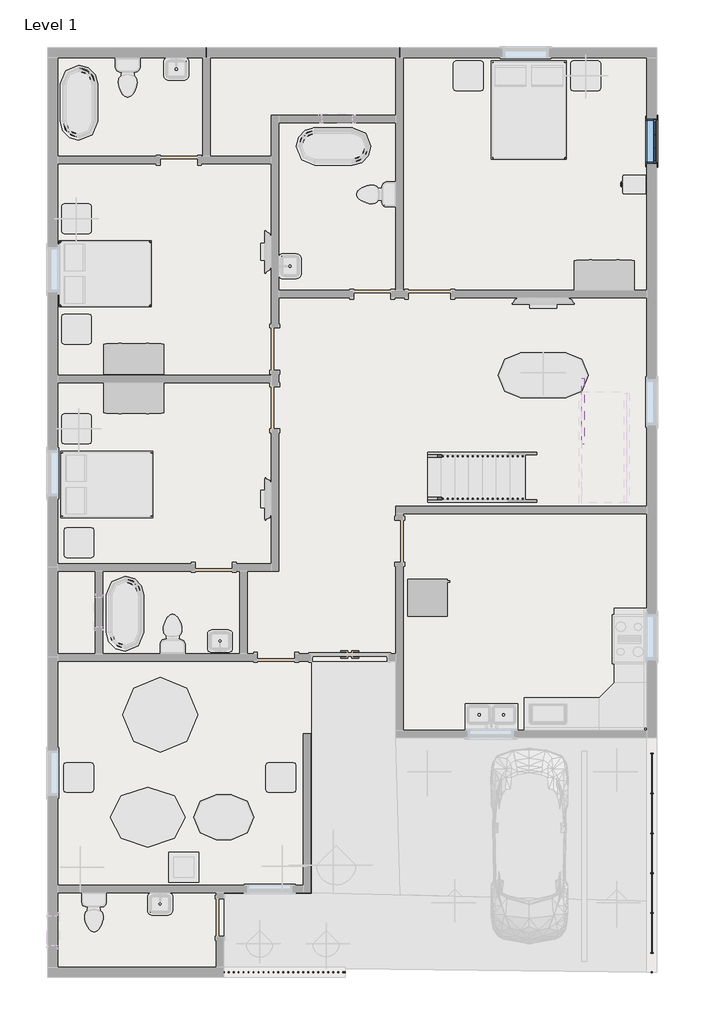
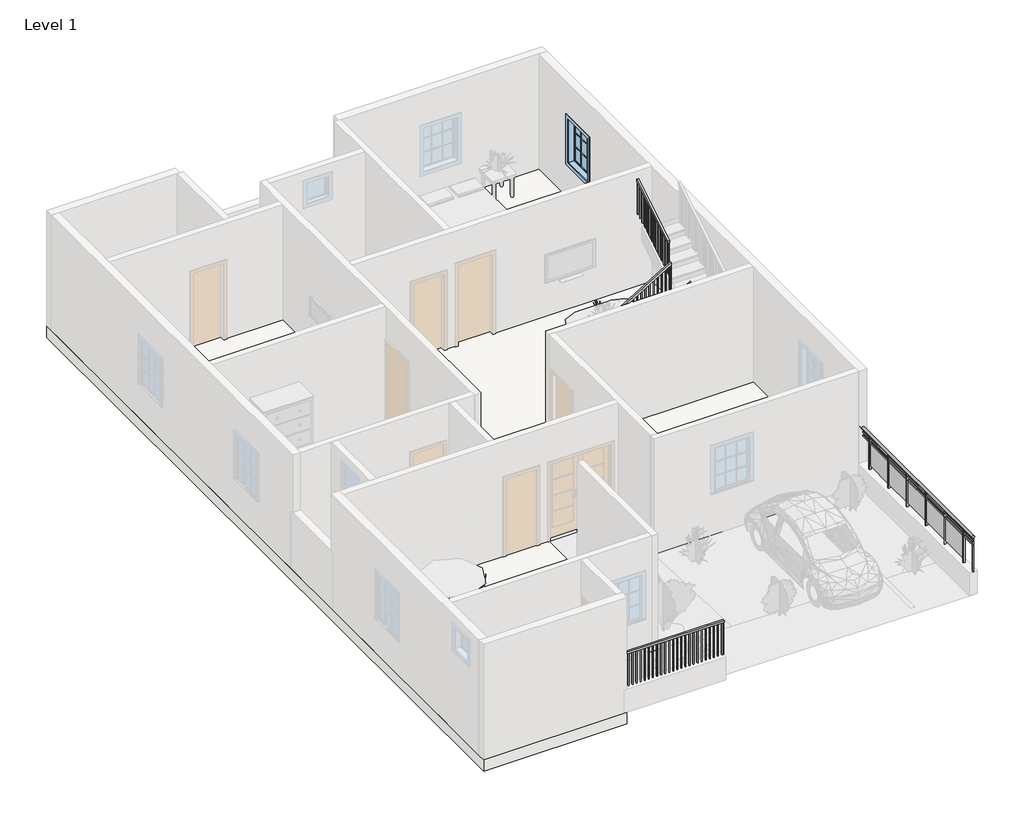
# One storey, part 2 of 3: 5 railings, 1 slab, 1 window.
"""IFC4 building model written with IfcOpenShell, lengths in millimetres."""

from ifc_helpers import new_model, si_unit, point, frame, origin, place, context, project, spatial, polyline, ellipse_curve, trimmed, outline, extrude, transform, mapped, element, save
from ifc_brep_helpers import plane_surface, extruded_surface, advanced_brep
from components import window_29c06734

model = new_model("IFC4")

# Units and contexts
model_context = context("Model", 3, world=origin())
ifc_project = project(units=[si_unit("LENGTHUNIT", "METRE", prefix="MILLI")], contexts=[model_context])

# Site, building, storey
site = spatial("IfcSite", under=ifc_project)
building = spatial("IfcBuilding", under=site)
storey = spatial("IfcBuildingStorey", under=building, Name="Level 1", Elevation=0.0)

# Railings
placement = place(None, origin())
element("IfcRailing", 1, ObjectType="Glass Panel - Bottom Fill", at=placement, inside=storey, context=model_context, shape_type="SolidModel", body=[
    advanced_brep(
    [(197.4210483, -2774.2231522, 1524.0), (121.2210483, -2774.2231522, 1524.0), (197.4210483, -7625.6231522, 1524.0), (121.2210483, -7625.6231522, 1524.0)],
    [
        (0, 1, ellipse_curve(frame((159.3210483, -2774.2231522, 1524.0), z_axis=(0.0, 1.0, 0.0), x_axis=(-1.0, 0.0, 0.0)), 38.1, 28.575)),
        (1, 0, ellipse_curve(frame((159.3210483, -2774.2231522, 1524.0), z_axis=(0.0, 1.0, 0.0), x_axis=(-1.0, 0.0, 0.0)), 38.1, 28.575)),
        (2, 3, ellipse_curve(frame((159.3210483, -7625.6231522, 1524.0), z_axis=(0.0, -1.0, 0.0), x_axis=(-1.0, 0.0, 0.0)), 38.1, 28.575)),
        (3, 2, ellipse_curve(frame((159.3210483, -7625.6231522, 1524.0), z_axis=(0.0, -1.0, 0.0), x_axis=(-1.0, 0.0, 0.0)), 38.1, 28.575)),
        (0, 2),
        (3, 1),
    ],
    [
        plane_surface(frame((159.3210483, -2774.2231522, 1524.0), z_axis=(0.0, 1.0, 0.0), x_axis=(0.0, 0.0, -1.0))),
        plane_surface(frame((159.3210483, -7625.6231522, 1524.0), z_axis=(0.0, -1.0, 0.0), x_axis=(0.0, 0.0, -1.0))),
        extruded_surface(trimmed(ellipse_curve(frame((159.3210483, -7625.6231522, 1524.0), z_axis=(0.0, 1.0, 0.0), x_axis=(-1.0, 0.0, 0.0)), 38.1, 28.575), [point((197.4210483, -7625.6231522, 1524.0))], [point((121.2210483, -7625.6231522, 1524.0))], True, "CARTESIAN"), (0.0, 4851.4, 0.0), 4851.4),
        extruded_surface(trimmed(ellipse_curve(frame((159.3210483, -7625.6231522, 1524.0), z_axis=(0.0, 1.0, 0.0), x_axis=(-1.0, 0.0, 0.0)), 38.1, 28.575), [point((121.2210483, -7625.6231522, 1524.0))], [point((197.4210483, -7625.6231522, 1524.0))], True, "CARTESIAN"), (0.0, 4851.4, 0.0), 4851.4),
    ],
    [
        (0, [[1, 2]]),
        (1, [[3, 4]]),
        (2, [[-1, 5, -4, 6]]),
        (3, [[-2, -6, -3, -5]]),
    ],
),
    extrude(outline(polyline([(146.6210483, -2774.2231522), (172.0210483, -2774.2231522), (172.0210483, -7625.6231522), (146.6210483, -7625.6231522), (146.6210483, -2774.2231522)])), frame((0.0, 0.0, 1409.7), z_axis=(0.0, 0.0, 1.0), x_axis=(1.0, 0.0, 0.0)), (0.0, 0.0, 1.0), 25.4),
    extrude(outline(polyline([(146.6210483, -2774.2231522), (172.0210483, -2774.2231522), (172.0210483, -7625.6231522), (146.6210483, -7625.6231522), (146.6210483, -2774.2231522)])), frame((0.0, 0.0, 1308.1), z_axis=(0.0, 0.0, 1.0), x_axis=(1.0, 0.0, 0.0)), (0.0, 0.0, 1.0), 25.4),
    extrude(outline(polyline([(133.9210483, -7225.5731522), (184.7210483, -7225.5731522), (184.7210483, -7238.2731522), (133.9210483, -7238.2731522), (133.9210483, -7225.5731522)])), frame((0.0, 0.0, 609.6), z_axis=(0.0, 0.0, 1.0), x_axis=(1.0, 0.0, 0.0)), (0.0, 0.0, 1.0), 885.6788223),
    extrude(outline(polyline([(165.8562053, -6419.1231522), (165.8562053, -7231.9231522), (159.5062053, -7231.9231522), (159.5062053, -6419.1231522), (165.8562053, -6419.1231522)])), frame((0.0, 0.0, 711.2), z_axis=(0.0, 0.0, 1.0), x_axis=(1.0, 0.0, 0.0)), (0.0, 0.0, 1.0), 596.9),
    extrude(outline(polyline([(133.9210483, -6412.7731522), (184.7210483, -6412.7731522), (184.7210483, -6425.4731522), (133.9210483, -6425.4731522), (133.9210483, -6412.7731522)])), frame((0.0, 0.0, 609.6), z_axis=(0.0, 0.0, 1.0), x_axis=(1.0, 0.0, 0.0)), (0.0, 0.0, 1.0), 885.6788223),
    extrude(outline(polyline([(165.8562053, -5606.3231522), (165.8562053, -6419.1231522), (159.5062053, -6419.1231522), (159.5062053, -5606.3231522), (165.8562053, -5606.3231522)])), frame((0.0, 0.0, 711.2), z_axis=(0.0, 0.0, 1.0), x_axis=(1.0, 0.0, 0.0)), (0.0, 0.0, 1.0), 596.9),
    extrude(outline(polyline([(133.9210483, -5599.9731522), (184.7210483, -5599.9731522), (184.7210483, -5612.6731522), (133.9210483, -5612.6731522), (133.9210483, -5599.9731522)])), frame((0.0, 0.0, 609.6), z_axis=(0.0, 0.0, 1.0), x_axis=(1.0, 0.0, 0.0)), (0.0, 0.0, 1.0), 885.6788223),
    extrude(outline(polyline([(165.8562053, -4793.5231522), (165.8562053, -5606.3231522), (159.5062053, -5606.3231522), (159.5062053, -4793.5231522), (165.8562053, -4793.5231522)])), frame((0.0, 0.0, 711.2), z_axis=(0.0, 0.0, 1.0), x_axis=(1.0, 0.0, 0.0)), (0.0, 0.0, 1.0), 596.9),
    extrude(outline(polyline([(133.9210483, -4787.1731522), (184.7210483, -4787.1731522), (184.7210483, -4799.8731522), (133.9210483, -4799.8731522), (133.9210483, -4787.1731522)])), frame((0.0, 0.0, 609.6), z_axis=(0.0, 0.0, 1.0), x_axis=(1.0, 0.0, 0.0)), (0.0, 0.0, 1.0), 885.6788223),
    extrude(outline(polyline([(165.8562053, -3980.7231522), (165.8562053, -4793.5231522), (159.5062053, -4793.5231522), (159.5062053, -3980.7231522), (165.8562053, -3980.7231522)])), frame((0.0, 0.0, 711.2), z_axis=(0.0, 0.0, 1.0), x_axis=(1.0, 0.0, 0.0)), (0.0, 0.0, 1.0), 596.9),
    extrude(outline(polyline([(133.9210483, -3974.3731522), (184.7210483, -3974.3731522), (184.7210483, -3987.0731522), (133.9210483, -3987.0731522), (133.9210483, -3974.3731522)])), frame((0.0, 0.0, 609.6), z_axis=(0.0, 0.0, 1.0), x_axis=(1.0, 0.0, 0.0)), (0.0, 0.0, 1.0), 885.6788223),
    extrude(outline(polyline([(165.8562053, -3167.9231522), (165.8562053, -3980.7231522), (159.5062053, -3980.7231522), (159.5062053, -3167.9231522), (165.8562053, -3167.9231522)])), frame((0.0, 0.0, 711.2), z_axis=(0.0, 0.0, 1.0), x_axis=(1.0, 0.0, 0.0)), (0.0, 0.0, 1.0), 596.9),
    extrude(outline(polyline([(133.9210483, -3161.5731522), (184.7210483, -3161.5731522), (184.7210483, -3174.2731522), (133.9210483, -3174.2731522), (133.9210483, -3161.5731522)])), frame((0.0, 0.0, 609.6), z_axis=(0.0, 0.0, 1.0), x_axis=(1.0, 0.0, 0.0)), (0.0, 0.0, 1.0), 885.6788223),
    extrude(outline(polyline([(149.7960483, -7612.9231522), (168.8460483, -7612.9231522), (168.8460483, -7631.9731522), (149.7960483, -7631.9731522), (149.7960483, -7612.9231522)])), frame((0.0, 0.0, 609.6), z_axis=(0.0, 0.0, 1.0), x_axis=(1.0, 0.0, 0.0)), (0.0, 0.0, 1.0), 885.6788223),
    extrude(outline(polyline([(149.7960483, -2767.8731522), (168.8460483, -2767.8731522), (168.8460483, -2786.9231522), (149.7960483, -2786.9231522), (149.7960483, -2767.8731522)])), frame((0.0, 0.0, 609.6), z_axis=(0.0, 0.0, 1.0), x_axis=(1.0, 0.0, 0.0)), (0.0, 0.0, 1.0), 885.6788223),
])
element("IfcRailing", 2, ObjectType="Handrail - Rectangular", at=placement, inside=storey, context=model_context, shape_type="SweptSolid", body=[
    extrude(outline(polyline([(1083.7333333, -4400.7663486), (1024.3318731, -4400.7663486), (2886.9985397, -1327.3663486), (2946.4, -1327.3663486), (1083.7333333, -4400.7663486)])), frame((0.0, 1993.3117215, 0.0), z_axis=(0.0, 1.0, 0.0), x_axis=(0.0, 0.0, 1.0)), (0.0, 0.0, 1.0), 50.8),
    extrude(outline(polyline([(2877.3773276, -1343.2413486), (2865.8318731, -1362.2913486), (1862.6666667, -1362.2913486), (1862.6666667, -1343.2413486), (2877.3773276, -1343.2413486)])), frame((0.0, 2009.1867215, 0.0), z_axis=(0.0, 1.0, 0.0), x_axis=(0.0, 0.0, 1.0)), (0.0, 0.0, 1.0), 19.05),
    extrude(outline(polyline([(2815.80157, -1444.8413486), (2804.2561155, -1463.8913486), (1862.6666667, -1463.8913486), (1862.6666667, -1444.8413486), (2815.80157, -1444.8413486)])), frame((0.0, 2009.1867215, 0.0), z_axis=(0.0, 1.0, 0.0), x_axis=(0.0, 0.0, 1.0)), (0.0, 0.0, 1.0), 19.05),
    extrude(outline(polyline([(2754.2258125, -1546.4413486), (2742.6803579, -1565.4913486), (1862.6666667, -1565.4913486), (1862.6666667, -1546.4413486), (2754.2258125, -1546.4413486)])), frame((0.0, 2009.1867215, 0.0), z_axis=(0.0, 1.0, 0.0), x_axis=(0.0, 0.0, 1.0)), (0.0, 0.0, 1.0), 19.05),
    extrude(outline(polyline([(2692.6500549, -1648.0413486), (2681.1046004, -1667.0913486), (1693.3333333, -1667.0913486), (1693.3333333, -1648.0413486), (2692.6500549, -1648.0413486)])), frame((0.0, 2009.1867215, 0.0), z_axis=(0.0, 1.0, 0.0), x_axis=(0.0, 0.0, 1.0)), (0.0, 0.0, 1.0), 19.05),
    extrude(outline(polyline([(2631.0742973, -1749.6413486), (2619.5288428, -1768.6913486), (1693.3333333, -1768.6913486), (1693.3333333, -1749.6413486), (2631.0742973, -1749.6413486)])), frame((0.0, 2009.1867215, 0.0), z_axis=(0.0, 1.0, 0.0), x_axis=(0.0, 0.0, 1.0)), (0.0, 0.0, 1.0), 19.05),
    extrude(outline(polyline([(2569.4985397, -1851.2413486), (2557.9530852, -1870.2913486), (1693.3333333, -1870.2913486), (1693.3333333, -1851.2413486), (2569.4985397, -1851.2413486)])), frame((0.0, 2009.1867215, 0.0), z_axis=(0.0, 1.0, 0.0), x_axis=(0.0, 0.0, 1.0)), (0.0, 0.0, 1.0), 19.05),
    extrude(outline(polyline([(2507.9227822, -1952.8413486), (2496.3773276, -1971.8913486), (1524.0, -1971.8913486), (1524.0, -1952.8413486), (2507.9227822, -1952.8413486)])), frame((0.0, 2009.1867215, 0.0), z_axis=(0.0, 1.0, 0.0), x_axis=(0.0, 0.0, 1.0)), (0.0, 0.0, 1.0), 19.05),
    extrude(outline(polyline([(2446.3470246, -2054.4413486), (2434.80157, -2073.4913486), (1524.0, -2073.4913486), (1524.0, -2054.4413486), (2446.3470246, -2054.4413486)])), frame((0.0, 2009.1867215, 0.0), z_axis=(0.0, 1.0, 0.0), x_axis=(0.0, 0.0, 1.0)), (0.0, 0.0, 1.0), 19.05),
    extrude(outline(polyline([(2384.771267, -2156.0413486), (2373.2258125, -2175.0913486), (1524.0, -2175.0913486), (1524.0, -2156.0413486), (2384.771267, -2156.0413486)])), frame((0.0, 2009.1867215, 0.0), z_axis=(0.0, 1.0, 0.0), x_axis=(0.0, 0.0, 1.0)), (0.0, 0.0, 1.0), 19.05),
    extrude(outline(polyline([(2323.1955094, -2257.6413486), (2311.6500549, -2276.6913486), (1354.6666667, -2276.6913486), (1354.6666667, -2257.6413486), (2323.1955094, -2257.6413486)])), frame((0.0, 2009.1867215, 0.0), z_axis=(0.0, 1.0, 0.0), x_axis=(0.0, 0.0, 1.0)), (0.0, 0.0, 1.0), 19.05),
    extrude(outline(polyline([(2261.6197519, -2359.2413486), (2250.0742973, -2378.2913486), (1354.6666667, -2378.2913486), (1354.6666667, -2359.2413486), (2261.6197519, -2359.2413486)])), frame((0.0, 2009.1867215, 0.0), z_axis=(0.0, 1.0, 0.0), x_axis=(0.0, 0.0, 1.0)), (0.0, 0.0, 1.0), 19.05),
    extrude(outline(polyline([(2200.0439943, -2460.8413486), (2188.4985397, -2479.8913486), (1185.3333333, -2479.8913486), (1185.3333333, -2460.8413486), (2200.0439943, -2460.8413486)])), frame((0.0, 2009.1867215, 0.0), z_axis=(0.0, 1.0, 0.0), x_axis=(0.0, 0.0, 1.0)), (0.0, 0.0, 1.0), 19.05),
    extrude(outline(polyline([(2138.4682367, -2562.4413486), (2126.9227822, -2581.4913486), (1185.3333333, -2581.4913486), (1185.3333333, -2562.4413486), (2138.4682367, -2562.4413486)])), frame((0.0, 2009.1867215, 0.0), z_axis=(0.0, 1.0, 0.0), x_axis=(0.0, 0.0, 1.0)), (0.0, 0.0, 1.0), 19.05),
    extrude(outline(polyline([(2076.8924791, -2664.0413486), (2065.3470246, -2683.0913486), (1185.3333333, -2683.0913486), (1185.3333333, -2664.0413486), (2076.8924791, -2664.0413486)])), frame((0.0, 2009.1867215, 0.0), z_axis=(0.0, 1.0, 0.0), x_axis=(0.0, 0.0, 1.0)), (0.0, 0.0, 1.0), 19.05),
    extrude(outline(polyline([(2015.3167216, -2765.6413486), (2003.771267, -2784.6913486), (1016.0, -2784.6913486), (1016.0, -2765.6413486), (2015.3167216, -2765.6413486)])), frame((0.0, 2009.1867215, 0.0), z_axis=(0.0, 1.0, 0.0), x_axis=(0.0, 0.0, 1.0)), (0.0, 0.0, 1.0), 19.05),
    extrude(outline(polyline([(1953.740964, -2867.2413486), (1942.1955094, -2886.2913486), (1016.0, -2886.2913486), (1016.0, -2867.2413486), (1953.740964, -2867.2413486)])), frame((0.0, 2009.1867215, 0.0), z_axis=(0.0, 1.0, 0.0), x_axis=(0.0, 0.0, 1.0)), (0.0, 0.0, 1.0), 19.05),
    extrude(outline(polyline([(1892.1652064, -2968.8413486), (1880.6197519, -2987.8913486), (1016.0, -2987.8913486), (1016.0, -2968.8413486), (1892.1652064, -2968.8413486)])), frame((0.0, 2009.1867215, 0.0), z_axis=(0.0, 1.0, 0.0), x_axis=(0.0, 0.0, 1.0)), (0.0, 0.0, 1.0), 19.05),
    extrude(outline(polyline([(1830.5894488, -3070.4413486), (1819.0439943, -3089.4913486), (846.6666667, -3089.4913486), (846.6666667, -3070.4413486), (1830.5894488, -3070.4413486)])), frame((0.0, 2009.1867215, 0.0), z_axis=(0.0, 1.0, 0.0), x_axis=(0.0, 0.0, 1.0)), (0.0, 0.0, 1.0), 19.05),
    extrude(outline(polyline([(1769.0136913, -3172.0413486), (1757.4682367, -3191.0913486), (846.6666667, -3191.0913486), (846.6666667, -3172.0413486), (1769.0136913, -3172.0413486)])), frame((0.0, 2009.1867215, 0.0), z_axis=(0.0, 1.0, 0.0), x_axis=(0.0, 0.0, 1.0)), (0.0, 0.0, 1.0), 19.05),
    extrude(outline(polyline([(1707.4379337, -3273.6413486), (1695.8924791, -3292.6913486), (846.6666667, -3292.6913486), (846.6666667, -3273.6413486), (1707.4379337, -3273.6413486)])), frame((0.0, 2009.1867215, 0.0), z_axis=(0.0, 1.0, 0.0), x_axis=(0.0, 0.0, 1.0)), (0.0, 0.0, 1.0), 19.05),
    extrude(outline(polyline([(1645.8621761, -3375.2413486), (1634.3167216, -3394.2913486), (677.3333333, -3394.2913486), (677.3333333, -3375.2413486), (1645.8621761, -3375.2413486)])), frame((0.0, 2009.1867215, 0.0), z_axis=(0.0, 1.0, 0.0), x_axis=(0.0, 0.0, 1.0)), (0.0, 0.0, 1.0), 19.05),
    extrude(outline(polyline([(1584.2864185, -3476.8413486), (1572.740964, -3495.8913486), (677.3333333, -3495.8913486), (677.3333333, -3476.8413486), (1584.2864185, -3476.8413486)])), frame((0.0, 2009.1867215, 0.0), z_axis=(0.0, 1.0, 0.0), x_axis=(0.0, 0.0, 1.0)), (0.0, 0.0, 1.0), 19.05),
    extrude(outline(polyline([(1522.710661, -3578.4413486), (1511.1652064, -3597.4913486), (508.0, -3597.4913486), (508.0, -3578.4413486), (1522.710661, -3578.4413486)])), frame((0.0, 2009.1867215, 0.0), z_axis=(0.0, 1.0, 0.0), x_axis=(0.0, 0.0, 1.0)), (0.0, 0.0, 1.0), 19.05),
    extrude(outline(polyline([(1461.1349034, -3680.0413486), (1449.5894488, -3699.0913486), (508.0, -3699.0913486), (508.0, -3680.0413486), (1461.1349034, -3680.0413486)])), frame((0.0, 2009.1867215, 0.0), z_axis=(0.0, 1.0, 0.0), x_axis=(0.0, 0.0, 1.0)), (0.0, 0.0, 1.0), 19.05),
    extrude(outline(polyline([(1399.5591458, -3781.6413486), (1388.0136913, -3800.6913486), (508.0, -3800.6913486), (508.0, -3781.6413486), (1399.5591458, -3781.6413486)])), frame((0.0, 2009.1867215, 0.0), z_axis=(0.0, 1.0, 0.0), x_axis=(0.0, 0.0, 1.0)), (0.0, 0.0, 1.0), 19.05),
    extrude(outline(polyline([(1337.9833882, -3883.2413486), (1326.4379337, -3902.2913486), (338.6666667, -3902.2913486), (338.6666667, -3883.2413486), (1337.9833882, -3883.2413486)])), frame((0.0, 2009.1867215, 0.0), z_axis=(0.0, 1.0, 0.0), x_axis=(0.0, 0.0, 1.0)), (0.0, 0.0, 1.0), 19.05),
    extrude(outline(polyline([(1276.4076307, -3984.8413486), (1264.8621761, -4003.8913486), (338.6666667, -4003.8913486), (338.6666667, -3984.8413486), (1276.4076307, -3984.8413486)])), frame((0.0, 2009.1867215, 0.0), z_axis=(0.0, 1.0, 0.0), x_axis=(0.0, 0.0, 1.0)), (0.0, 0.0, 1.0), 19.05),
    extrude(outline(polyline([(1214.8318731, -4086.4413486), (1203.2864185, -4105.4913486), (338.6666667, -4105.4913486), (338.6666667, -4086.4413486), (1214.8318731, -4086.4413486)])), frame((0.0, 2009.1867215, 0.0), z_axis=(0.0, 1.0, 0.0), x_axis=(0.0, 0.0, 1.0)), (0.0, 0.0, 1.0), 19.05),
    extrude(outline(polyline([(1153.2561155, -4188.0413486), (1141.710661, -4207.0913486), (169.3333333, -4207.0913486), (169.3333333, -4188.0413486), (1153.2561155, -4188.0413486)])), frame((0.0, 2009.1867215, 0.0), z_axis=(0.0, 1.0, 0.0), x_axis=(0.0, 0.0, 1.0)), (0.0, 0.0, 1.0), 19.05),
    extrude(outline(polyline([(1091.6803579, -4289.6413486), (1080.1349034, -4308.6913486), (169.3333333, -4308.6913486), (169.3333333, -4289.6413486), (1091.6803579, -4289.6413486)])), frame((0.0, 2009.1867215, 0.0), z_axis=(0.0, 1.0, 0.0), x_axis=(0.0, 0.0, 1.0)), (0.0, 0.0, 1.0), 19.05),
    extrude(outline(polyline([(2886.9985397, -1327.3663486), (2875.4530852, -1346.4163486), (1862.6666667, -1346.4163486), (1862.6666667, -1327.3663486), (2886.9985397, -1327.3663486)])), frame((0.0, 2009.1867215, 0.0), z_axis=(0.0, 1.0, 0.0), x_axis=(0.0, 0.0, 1.0)), (0.0, 0.0, 1.0), 19.05),
    extrude(outline(polyline([(1035.8773276, -4381.7163486), (1024.3318731, -4400.7663486), (169.3333333, -4400.7663486), (169.3333333, -4381.7163486), (1035.8773276, -4381.7163486)])), frame((0.0, 2009.1867215, 0.0), z_axis=(0.0, 1.0, 0.0), x_axis=(0.0, 0.0, 1.0)), (0.0, 0.0, 1.0), 19.05),
])
element("IfcRailing", 3, ObjectType="Handrail - Rectangular", at=placement, inside=storey, context=model_context, shape_type="SweptSolid", body=[
    extrude(outline(polyline([(1083.7333333, -4400.7663486), (1024.3318731, -4400.7663486), (2886.9985397, -1327.3663486), (2946.4, -1327.3663486), (1083.7333333, -4400.7663486)])), frame((0.0, 2856.9117215, 0.0), z_axis=(0.0, 1.0, 0.0), x_axis=(0.0, 0.0, 1.0)), (0.0, 0.0, 1.0), 50.8),
    extrude(outline(polyline([(2865.8318731, -1362.2913486), (1862.6666667, -1362.2913486), (1862.6666667, -1343.2413486), (2877.3773276, -1343.2413486), (2865.8318731, -1362.2913486)])), frame((0.0, 2872.7867215, 0.0), z_axis=(0.0, 1.0, 0.0), x_axis=(0.0, 0.0, 1.0)), (0.0, 0.0, 1.0), 19.05),
    extrude(outline(polyline([(2804.2561155, -1463.8913486), (1862.6666667, -1463.8913486), (1862.6666667, -1444.8413486), (2815.80157, -1444.8413486), (2804.2561155, -1463.8913486)])), frame((0.0, 2872.7867215, 0.0), z_axis=(0.0, 1.0, 0.0), x_axis=(0.0, 0.0, 1.0)), (0.0, 0.0, 1.0), 19.05),
    extrude(outline(polyline([(2742.6803579, -1565.4913486), (1862.6666667, -1565.4913486), (1862.6666667, -1546.4413486), (2754.2258125, -1546.4413486), (2742.6803579, -1565.4913486)])), frame((0.0, 2872.7867215, 0.0), z_axis=(0.0, 1.0, 0.0), x_axis=(0.0, 0.0, 1.0)), (0.0, 0.0, 1.0), 19.05),
    extrude(outline(polyline([(2681.1046004, -1667.0913486), (1693.3333333, -1667.0913486), (1693.3333333, -1648.0413486), (2692.6500549, -1648.0413486), (2681.1046004, -1667.0913486)])), frame((0.0, 2872.7867215, 0.0), z_axis=(0.0, 1.0, 0.0), x_axis=(0.0, 0.0, 1.0)), (0.0, 0.0, 1.0), 19.05),
    extrude(outline(polyline([(2619.5288428, -1768.6913486), (1693.3333333, -1768.6913486), (1693.3333333, -1749.6413486), (2631.0742973, -1749.6413486), (2619.5288428, -1768.6913486)])), frame((0.0, 2872.7867215, 0.0), z_axis=(0.0, 1.0, 0.0), x_axis=(0.0, 0.0, 1.0)), (0.0, 0.0, 1.0), 19.05),
    extrude(outline(polyline([(2557.9530852, -1870.2913486), (1693.3333333, -1870.2913486), (1693.3333333, -1851.2413486), (2569.4985397, -1851.2413486), (2557.9530852, -1870.2913486)])), frame((0.0, 2872.7867215, 0.0), z_axis=(0.0, 1.0, 0.0), x_axis=(0.0, 0.0, 1.0)), (0.0, 0.0, 1.0), 19.05),
    extrude(outline(polyline([(2496.3773276, -1971.8913486), (1524.0, -1971.8913486), (1524.0, -1952.8413486), (2507.9227822, -1952.8413486), (2496.3773276, -1971.8913486)])), frame((0.0, 2872.7867215, 0.0), z_axis=(0.0, 1.0, 0.0), x_axis=(0.0, 0.0, 1.0)), (0.0, 0.0, 1.0), 19.05),
    extrude(outline(polyline([(2434.80157, -2073.4913486), (1524.0, -2073.4913486), (1524.0, -2054.4413486), (2446.3470246, -2054.4413486), (2434.80157, -2073.4913486)])), frame((0.0, 2872.7867215, 0.0), z_axis=(0.0, 1.0, 0.0), x_axis=(0.0, 0.0, 1.0)), (0.0, 0.0, 1.0), 19.05),
    extrude(outline(polyline([(2373.2258125, -2175.0913486), (1524.0, -2175.0913486), (1524.0, -2156.0413486), (2384.771267, -2156.0413486), (2373.2258125, -2175.0913486)])), frame((0.0, 2872.7867215, 0.0), z_axis=(0.0, 1.0, 0.0), x_axis=(0.0, 0.0, 1.0)), (0.0, 0.0, 1.0), 19.05),
    extrude(outline(polyline([(2311.6500549, -2276.6913486), (1354.6666667, -2276.6913486), (1354.6666667, -2257.6413486), (2323.1955094, -2257.6413486), (2311.6500549, -2276.6913486)])), frame((0.0, 2872.7867215, 0.0), z_axis=(0.0, 1.0, 0.0), x_axis=(0.0, 0.0, 1.0)), (0.0, 0.0, 1.0), 19.05),
    extrude(outline(polyline([(2250.0742973, -2378.2913486), (1354.6666667, -2378.2913486), (1354.6666667, -2359.2413486), (2261.6197519, -2359.2413486), (2250.0742973, -2378.2913486)])), frame((0.0, 2872.7867215, 0.0), z_axis=(0.0, 1.0, 0.0), x_axis=(0.0, 0.0, 1.0)), (0.0, 0.0, 1.0), 19.05),
    extrude(outline(polyline([(2188.4985397, -2479.8913486), (1185.3333333, -2479.8913486), (1185.3333333, -2460.8413486), (2200.0439943, -2460.8413486), (2188.4985397, -2479.8913486)])), frame((0.0, 2872.7867215, 0.0), z_axis=(0.0, 1.0, 0.0), x_axis=(0.0, 0.0, 1.0)), (0.0, 0.0, 1.0), 19.05),
    extrude(outline(polyline([(2126.9227822, -2581.4913486), (1185.3333333, -2581.4913486), (1185.3333333, -2562.4413486), (2138.4682367, -2562.4413486), (2126.9227822, -2581.4913486)])), frame((0.0, 2872.7867215, 0.0), z_axis=(0.0, 1.0, 0.0), x_axis=(0.0, 0.0, 1.0)), (0.0, 0.0, 1.0), 19.05),
    extrude(outline(polyline([(2065.3470246, -2683.0913486), (1185.3333333, -2683.0913486), (1185.3333333, -2664.0413486), (2076.8924791, -2664.0413486), (2065.3470246, -2683.0913486)])), frame((0.0, 2872.7867215, 0.0), z_axis=(0.0, 1.0, 0.0), x_axis=(0.0, 0.0, 1.0)), (0.0, 0.0, 1.0), 19.05),
    extrude(outline(polyline([(2003.771267, -2784.6913486), (1016.0, -2784.6913486), (1016.0, -2765.6413486), (2015.3167216, -2765.6413486), (2003.771267, -2784.6913486)])), frame((0.0, 2872.7867215, 0.0), z_axis=(0.0, 1.0, 0.0), x_axis=(0.0, 0.0, 1.0)), (0.0, 0.0, 1.0), 19.05),
    extrude(outline(polyline([(1942.1955094, -2886.2913486), (1016.0, -2886.2913486), (1016.0, -2867.2413486), (1953.740964, -2867.2413486), (1942.1955094, -2886.2913486)])), frame((0.0, 2872.7867215, 0.0), z_axis=(0.0, 1.0, 0.0), x_axis=(0.0, 0.0, 1.0)), (0.0, 0.0, 1.0), 19.05),
    extrude(outline(polyline([(1880.6197519, -2987.8913486), (1016.0, -2987.8913486), (1016.0, -2968.8413486), (1892.1652064, -2968.8413486), (1880.6197519, -2987.8913486)])), frame((0.0, 2872.7867215, 0.0), z_axis=(0.0, 1.0, 0.0), x_axis=(0.0, 0.0, 1.0)), (0.0, 0.0, 1.0), 19.05),
    extrude(outline(polyline([(1819.0439943, -3089.4913486), (846.6666667, -3089.4913486), (846.6666667, -3070.4413486), (1830.5894488, -3070.4413486), (1819.0439943, -3089.4913486)])), frame((0.0, 2872.7867215, 0.0), z_axis=(0.0, 1.0, 0.0), x_axis=(0.0, 0.0, 1.0)), (0.0, 0.0, 1.0), 19.05),
    extrude(outline(polyline([(1757.4682367, -3191.0913486), (846.6666667, -3191.0913486), (846.6666667, -3172.0413486), (1769.0136913, -3172.0413486), (1757.4682367, -3191.0913486)])), frame((0.0, 2872.7867215, 0.0), z_axis=(0.0, 1.0, 0.0), x_axis=(0.0, 0.0, 1.0)), (0.0, 0.0, 1.0), 19.05),
    extrude(outline(polyline([(1695.8924791, -3292.6913486), (846.6666667, -3292.6913486), (846.6666667, -3273.6413486), (1707.4379337, -3273.6413486), (1695.8924791, -3292.6913486)])), frame((0.0, 2872.7867215, 0.0), z_axis=(0.0, 1.0, 0.0), x_axis=(0.0, 0.0, 1.0)), (0.0, 0.0, 1.0), 19.05),
    extrude(outline(polyline([(1634.3167216, -3394.2913486), (677.3333333, -3394.2913486), (677.3333333, -3375.2413486), (1645.8621761, -3375.2413486), (1634.3167216, -3394.2913486)])), frame((0.0, 2872.7867215, 0.0), z_axis=(0.0, 1.0, 0.0), x_axis=(0.0, 0.0, 1.0)), (0.0, 0.0, 1.0), 19.05),
    extrude(outline(polyline([(1572.740964, -3495.8913486), (677.3333333, -3495.8913486), (677.3333333, -3476.8413486), (1584.2864185, -3476.8413486), (1572.740964, -3495.8913486)])), frame((0.0, 2872.7867215, 0.0), z_axis=(0.0, 1.0, 0.0), x_axis=(0.0, 0.0, 1.0)), (0.0, 0.0, 1.0), 19.05),
    extrude(outline(polyline([(1511.1652064, -3597.4913486), (508.0, -3597.4913486), (508.0, -3578.4413486), (1522.710661, -3578.4413486), (1511.1652064, -3597.4913486)])), frame((0.0, 2872.7867215, 0.0), z_axis=(0.0, 1.0, 0.0), x_axis=(0.0, 0.0, 1.0)), (0.0, 0.0, 1.0), 19.05),
    extrude(outline(polyline([(1449.5894488, -3699.0913486), (508.0, -3699.0913486), (508.0, -3680.0413486), (1461.1349034, -3680.0413486), (1449.5894488, -3699.0913486)])), frame((0.0, 2872.7867215, 0.0), z_axis=(0.0, 1.0, 0.0), x_axis=(0.0, 0.0, 1.0)), (0.0, 0.0, 1.0), 19.05),
    extrude(outline(polyline([(1388.0136913, -3800.6913486), (508.0, -3800.6913486), (508.0, -3781.6413486), (1399.5591458, -3781.6413486), (1388.0136913, -3800.6913486)])), frame((0.0, 2872.7867215, 0.0), z_axis=(0.0, 1.0, 0.0), x_axis=(0.0, 0.0, 1.0)), (0.0, 0.0, 1.0), 19.05),
    extrude(outline(polyline([(1326.4379337, -3902.2913486), (338.6666667, -3902.2913486), (338.6666667, -3883.2413486), (1337.9833882, -3883.2413486), (1326.4379337, -3902.2913486)])), frame((0.0, 2872.7867215, 0.0), z_axis=(0.0, 1.0, 0.0), x_axis=(0.0, 0.0, 1.0)), (0.0, 0.0, 1.0), 19.05),
    extrude(outline(polyline([(1264.8621761, -4003.8913486), (338.6666667, -4003.8913486), (338.6666667, -3984.8413486), (1276.4076307, -3984.8413486), (1264.8621761, -4003.8913486)])), frame((0.0, 2872.7867215, 0.0), z_axis=(0.0, 1.0, 0.0), x_axis=(0.0, 0.0, 1.0)), (0.0, 0.0, 1.0), 19.05),
    extrude(outline(polyline([(1203.2864185, -4105.4913486), (338.6666667, -4105.4913486), (338.6666667, -4086.4413486), (1214.8318731, -4086.4413486), (1203.2864185, -4105.4913486)])), frame((0.0, 2872.7867215, 0.0), z_axis=(0.0, 1.0, 0.0), x_axis=(0.0, 0.0, 1.0)), (0.0, 0.0, 1.0), 19.05),
    extrude(outline(polyline([(1141.710661, -4207.0913486), (169.3333333, -4207.0913486), (169.3333333, -4188.0413486), (1153.2561155, -4188.0413486), (1141.710661, -4207.0913486)])), frame((0.0, 2872.7867215, 0.0), z_axis=(0.0, 1.0, 0.0), x_axis=(0.0, 0.0, 1.0)), (0.0, 0.0, 1.0), 19.05),
    extrude(outline(polyline([(1080.1349034, -4308.6913486), (169.3333333, -4308.6913486), (169.3333333, -4289.6413486), (1091.6803579, -4289.6413486), (1080.1349034, -4308.6913486)])), frame((0.0, 2872.7867215, 0.0), z_axis=(0.0, 1.0, 0.0), x_axis=(0.0, 0.0, 1.0)), (0.0, 0.0, 1.0), 19.05),
    extrude(outline(polyline([(2875.4530852, -1346.4163486), (1862.6666667, -1346.4163486), (1862.6666667, -1327.3663486), (2886.9985397, -1327.3663486), (2875.4530852, -1346.4163486)])), frame((0.0, 2872.7867215, 0.0), z_axis=(0.0, 1.0, 0.0), x_axis=(0.0, 0.0, 1.0)), (0.0, 0.0, 1.0), 19.05),
    extrude(outline(polyline([(1024.3318731, -4400.7663486), (169.3333333, -4400.7663486), (169.3333333, -4381.7163486), (1035.8773276, -4381.7163486), (1024.3318731, -4400.7663486)])), frame((0.0, 2872.7867215, 0.0), z_axis=(0.0, 1.0, 0.0), x_axis=(0.0, 0.0, 1.0)), (0.0, 0.0, 1.0), 19.05),
])
element("IfcRailing", 4, ObjectType="Handrail - Rectangular", at=placement, inside=storey, context=model_context, shape_type="SweptSolid", body=[
    extrude(outline(polyline([(3124.388941, 3271.7078476), (3124.388941, 3331.1093079), (4470.588941, 4146.9880957), (4470.588941, 4087.5866355), (3124.388941, 3271.7078476)])), frame((-1263.0789517, 0.0, 0.0), z_axis=(1.0, 0.0, 0.0), x_axis=(0.0, 1.0, 0.0)), (0.0, 0.0, 1.0), 50.8),
    extrude(outline(polyline([(3140.263941, 3281.4682367), (3159.313941, 3293.0136913), (3159.313941, 2370.6666667), (3140.263941, 2370.6666667), (3140.263941, 3281.4682367)])), frame((-1247.2039517, 0.0, 0.0), z_axis=(1.0, 0.0, 0.0), x_axis=(0.0, 1.0, 0.0)), (0.0, 0.0, 1.0), 19.05),
    extrude(outline(polyline([(3241.863941, 3343.0439943), (3260.913941, 3354.5894488), (3260.913941, 2370.6666667), (3241.863941, 2370.6666667), (3241.863941, 3343.0439943)])), frame((-1247.2039517, 0.0, 0.0), z_axis=(1.0, 0.0, 0.0), x_axis=(0.0, 1.0, 0.0)), (0.0, 0.0, 1.0), 19.05),
    extrude(outline(polyline([(3343.463941, 3404.6197519), (3362.513941, 3416.1652064), (3362.513941, 2540.0), (3343.463941, 2540.0), (3343.463941, 3404.6197519)])), frame((-1247.2039517, 0.0, 0.0), z_axis=(1.0, 0.0, 0.0), x_axis=(0.0, 1.0, 0.0)), (0.0, 0.0, 1.0), 19.05),
    extrude(outline(polyline([(3445.063941, 3466.1955094), (3464.113941, 3477.740964), (3464.113941, 2540.0), (3445.063941, 2540.0), (3445.063941, 3466.1955094)])), frame((-1247.2039517, 0.0, 0.0), z_axis=(1.0, 0.0, 0.0), x_axis=(0.0, 1.0, 0.0)), (0.0, 0.0, 1.0), 19.05),
    extrude(outline(polyline([(3546.663941, 3527.771267), (3565.713941, 3539.3167216), (3565.713941, 2540.0), (3546.663941, 2540.0), (3546.663941, 3527.771267)])), frame((-1247.2039517, 0.0, 0.0), z_axis=(1.0, 0.0, 0.0), x_axis=(0.0, 1.0, 0.0)), (0.0, 0.0, 1.0), 19.05),
    extrude(outline(polyline([(3648.263941, 3589.3470246), (3667.313941, 3600.8924791), (3667.313941, 2709.3333333), (3648.263941, 2709.3333333), (3648.263941, 3589.3470246)])), frame((-1247.2039517, 0.0, 0.0), z_axis=(1.0, 0.0, 0.0), x_axis=(0.0, 1.0, 0.0)), (0.0, 0.0, 1.0), 19.05),
    extrude(outline(polyline([(3749.863941, 3650.9227822), (3768.913941, 3662.4682367), (3768.913941, 2709.3333333), (3749.863941, 2709.3333333), (3749.863941, 3650.9227822)])), frame((-1247.2039517, 0.0, 0.0), z_axis=(1.0, 0.0, 0.0), x_axis=(0.0, 1.0, 0.0)), (0.0, 0.0, 1.0), 19.05),
    extrude(outline(polyline([(3851.463941, 3712.4985397), (3870.513941, 3724.0439943), (3870.513941, 2709.3333333), (3851.463941, 2709.3333333), (3851.463941, 3712.4985397)])), frame((-1247.2039517, 0.0, 0.0), z_axis=(1.0, 0.0, 0.0), x_axis=(0.0, 1.0, 0.0)), (0.0, 0.0, 1.0), 19.05),
    extrude(outline(polyline([(3953.063941, 3774.0742973), (3972.113941, 3785.6197519), (3972.113941, 2878.6666667), (3953.063941, 2878.6666667), (3953.063941, 3774.0742973)])), frame((-1247.2039517, 0.0, 0.0), z_axis=(1.0, 0.0, 0.0), x_axis=(0.0, 1.0, 0.0)), (0.0, 0.0, 1.0), 19.05),
    extrude(outline(polyline([(4054.663941, 3835.6500549), (4073.713941, 3847.1955094), (4073.713941, 2878.6666667), (4054.663941, 2878.6666667), (4054.663941, 3835.6500549)])), frame((-1247.2039517, 0.0, 0.0), z_axis=(1.0, 0.0, 0.0), x_axis=(0.0, 1.0, 0.0)), (0.0, 0.0, 1.0), 19.05),
    extrude(outline(polyline([(4156.263941, 3897.0866355), (4175.313941, 3908.63209), (4175.313941, 2878.6666667), (4156.263941, 2878.6666667), (4156.263941, 3897.0866355)])), frame((-1247.2039517, 0.0, 0.0), z_axis=(1.0, 0.0, 0.0), x_axis=(0.0, 1.0, 0.0)), (0.0, 0.0, 1.0), 19.05),
    extrude(outline(polyline([(4257.863941, 3958.6623931), (4276.913941, 3970.2078476), (4276.913941, 3109.4365806), (4257.863941, 3109.4365806), (4257.863941, 3958.6623931)])), frame((-1247.2039517, 0.0, 0.0), z_axis=(1.0, 0.0, 0.0), x_axis=(0.0, 1.0, 0.0)), (0.0, 0.0, 1.0), 19.05),
    extrude(outline(polyline([(4359.463941, 4020.2381506), (4378.513941, 4031.7836052), (4378.513941, 3171.0123382), (4359.463941, 3171.0123382), (4359.463941, 4020.2381506)])), frame((-1247.2039517, 0.0, 0.0), z_axis=(1.0, 0.0, 0.0), x_axis=(0.0, 1.0, 0.0)), (0.0, 0.0, 1.0), 19.05),
    extrude(outline(polyline([(3124.388941, 3271.7078476), (3143.438941, 3283.2533021), (3143.438941, 2370.6666667), (3124.388941, 2370.6666667), (3124.388941, 3271.7078476)])), frame((-1247.2039517, 0.0, 0.0), z_axis=(1.0, 0.0, 0.0), x_axis=(0.0, 1.0, 0.0)), (0.0, 0.0, 1.0), 19.05),
    extrude(outline(polyline([(4451.538941, 4076.0411809), (4470.588941, 4087.5866355), (4470.588941, 3226.8153685), (4451.538941, 3226.8153685), (4451.538941, 4076.0411809)])), frame((-1247.2039517, 0.0, 0.0), z_axis=(1.0, 0.0, 0.0), x_axis=(0.0, 1.0, 0.0)), (0.0, 0.0, 1.0), 19.05),
])
element("IfcRailing", 5, ObjectType="Handrail - Rectangular", at=placement, inside=storey, context=model_context, shape_type="SweptSolid", body=[
    extrude(outline(polyline([(-8556.6067873, -7651.0231522), (-8556.6067873, -7600.2231522), (-6079.5539517, -7600.2231522), (-6079.5539517, -7651.0231522), (-8556.6067873, -7651.0231522)])), frame((0.0, 0.0, 1473.2), z_axis=(0.0, 0.0, 1.0), x_axis=(1.0, 0.0, 0.0)), (0.0, 0.0, 1.0), 50.8),
    extrude(outline(polyline([(-6127.7317873, -7635.1481522), (-6127.7317873, -7616.0981522), (-6108.6817873, -7616.0981522), (-6108.6817873, -7635.1481522), (-6127.7317873, -7635.1481522)])), frame((0.0, 0.0, 609.6), z_axis=(0.0, 0.0, 1.0), x_axis=(1.0, 0.0, 0.0)), (0.0, 0.0, 1.0), 863.6),
    extrude(outline(polyline([(-6229.3317873, -7635.1481522), (-6229.3317873, -7616.0981522), (-6210.2817873, -7616.0981522), (-6210.2817873, -7635.1481522), (-6229.3317873, -7635.1481522)])), frame((0.0, 0.0, 609.6), z_axis=(0.0, 0.0, 1.0), x_axis=(1.0, 0.0, 0.0)), (0.0, 0.0, 1.0), 863.6),
    extrude(outline(polyline([(-6330.9317873, -7635.1481522), (-6330.9317873, -7616.0981522), (-6311.8817873, -7616.0981522), (-6311.8817873, -7635.1481522), (-6330.9317873, -7635.1481522)])), frame((0.0, 0.0, 609.6), z_axis=(0.0, 0.0, 1.0), x_axis=(1.0, 0.0, 0.0)), (0.0, 0.0, 1.0), 863.6),
    extrude(outline(polyline([(-6432.5317873, -7635.1481522), (-6432.5317873, -7616.0981522), (-6413.4817873, -7616.0981522), (-6413.4817873, -7635.1481522), (-6432.5317873, -7635.1481522)])), frame((0.0, 0.0, 609.6), z_axis=(0.0, 0.0, 1.0), x_axis=(1.0, 0.0, 0.0)), (0.0, 0.0, 1.0), 863.6),
    extrude(outline(polyline([(-6534.1317873, -7635.1481522), (-6534.1317873, -7616.0981522), (-6515.0817873, -7616.0981522), (-6515.0817873, -7635.1481522), (-6534.1317873, -7635.1481522)])), frame((0.0, 0.0, 609.6), z_axis=(0.0, 0.0, 1.0), x_axis=(1.0, 0.0, 0.0)), (0.0, 0.0, 1.0), 863.6),
    extrude(outline(polyline([(-6635.7317873, -7635.1481522), (-6635.7317873, -7616.0981522), (-6616.6817873, -7616.0981522), (-6616.6817873, -7635.1481522), (-6635.7317873, -7635.1481522)])), frame((0.0, 0.0, 609.6), z_axis=(0.0, 0.0, 1.0), x_axis=(1.0, 0.0, 0.0)), (0.0, 0.0, 1.0), 863.6),
    extrude(outline(polyline([(-6737.3317873, -7635.1481522), (-6737.3317873, -7616.0981522), (-6718.2817873, -7616.0981522), (-6718.2817873, -7635.1481522), (-6737.3317873, -7635.1481522)])), frame((0.0, 0.0, 609.6), z_axis=(0.0, 0.0, 1.0), x_axis=(1.0, 0.0, 0.0)), (0.0, 0.0, 1.0), 863.6),
    extrude(outline(polyline([(-6838.9317873, -7635.1481522), (-6838.9317873, -7616.0981522), (-6819.8817873, -7616.0981522), (-6819.8817873, -7635.1481522), (-6838.9317873, -7635.1481522)])), frame((0.0, 0.0, 609.6), z_axis=(0.0, 0.0, 1.0), x_axis=(1.0, 0.0, 0.0)), (0.0, 0.0, 1.0), 863.6),
    extrude(outline(polyline([(-6940.5317873, -7635.1481522), (-6940.5317873, -7616.0981522), (-6921.4817873, -7616.0981522), (-6921.4817873, -7635.1481522), (-6940.5317873, -7635.1481522)])), frame((0.0, 0.0, 609.6), z_axis=(0.0, 0.0, 1.0), x_axis=(1.0, 0.0, 0.0)), (0.0, 0.0, 1.0), 863.6),
    extrude(outline(polyline([(-7042.1317873, -7635.1481522), (-7042.1317873, -7616.0981522), (-7023.0817873, -7616.0981522), (-7023.0817873, -7635.1481522), (-7042.1317873, -7635.1481522)])), frame((0.0, 0.0, 609.6), z_axis=(0.0, 0.0, 1.0), x_axis=(1.0, 0.0, 0.0)), (0.0, 0.0, 1.0), 863.6),
    extrude(outline(polyline([(-7143.7317873, -7635.1481522), (-7143.7317873, -7616.0981522), (-7124.6817873, -7616.0981522), (-7124.6817873, -7635.1481522), (-7143.7317873, -7635.1481522)])), frame((0.0, 0.0, 609.6), z_axis=(0.0, 0.0, 1.0), x_axis=(1.0, 0.0, 0.0)), (0.0, 0.0, 1.0), 863.6),
    extrude(outline(polyline([(-7245.3317873, -7635.1481522), (-7245.3317873, -7616.0981522), (-7226.2817873, -7616.0981522), (-7226.2817873, -7635.1481522), (-7245.3317873, -7635.1481522)])), frame((0.0, 0.0, 609.6), z_axis=(0.0, 0.0, 1.0), x_axis=(1.0, 0.0, 0.0)), (0.0, 0.0, 1.0), 863.6),
    extrude(outline(polyline([(-7346.9317873, -7635.1481522), (-7346.9317873, -7616.0981522), (-7327.8817873, -7616.0981522), (-7327.8817873, -7635.1481522), (-7346.9317873, -7635.1481522)])), frame((0.0, 0.0, 609.6), z_axis=(0.0, 0.0, 1.0), x_axis=(1.0, 0.0, 0.0)), (0.0, 0.0, 1.0), 863.6),
    extrude(outline(polyline([(-7448.5317873, -7635.1481522), (-7448.5317873, -7616.0981522), (-7429.4817873, -7616.0981522), (-7429.4817873, -7635.1481522), (-7448.5317873, -7635.1481522)])), frame((0.0, 0.0, 609.6), z_axis=(0.0, 0.0, 1.0), x_axis=(1.0, 0.0, 0.0)), (0.0, 0.0, 1.0), 863.6),
    extrude(outline(polyline([(-7550.1317873, -7635.1481522), (-7550.1317873, -7616.0981522), (-7531.0817873, -7616.0981522), (-7531.0817873, -7635.1481522), (-7550.1317873, -7635.1481522)])), frame((0.0, 0.0, 609.6), z_axis=(0.0, 0.0, 1.0), x_axis=(1.0, 0.0, 0.0)), (0.0, 0.0, 1.0), 863.6),
    extrude(outline(polyline([(-7651.7317873, -7635.1481522), (-7651.7317873, -7616.0981522), (-7632.6817873, -7616.0981522), (-7632.6817873, -7635.1481522), (-7651.7317873, -7635.1481522)])), frame((0.0, 0.0, 609.6), z_axis=(0.0, 0.0, 1.0), x_axis=(1.0, 0.0, 0.0)), (0.0, 0.0, 1.0), 863.6),
    extrude(outline(polyline([(-7753.3317873, -7635.1481522), (-7753.3317873, -7616.0981522), (-7734.2817873, -7616.0981522), (-7734.2817873, -7635.1481522), (-7753.3317873, -7635.1481522)])), frame((0.0, 0.0, 609.6), z_axis=(0.0, 0.0, 1.0), x_axis=(1.0, 0.0, 0.0)), (0.0, 0.0, 1.0), 863.6),
    extrude(outline(polyline([(-7854.9317873, -7635.1481522), (-7854.9317873, -7616.0981522), (-7835.8817873, -7616.0981522), (-7835.8817873, -7635.1481522), (-7854.9317873, -7635.1481522)])), frame((0.0, 0.0, 609.6), z_axis=(0.0, 0.0, 1.0), x_axis=(1.0, 0.0, 0.0)), (0.0, 0.0, 1.0), 863.6),
    extrude(outline(polyline([(-7956.5317873, -7635.1481522), (-7956.5317873, -7616.0981522), (-7937.4817873, -7616.0981522), (-7937.4817873, -7635.1481522), (-7956.5317873, -7635.1481522)])), frame((0.0, 0.0, 609.6), z_axis=(0.0, 0.0, 1.0), x_axis=(1.0, 0.0, 0.0)), (0.0, 0.0, 1.0), 863.6),
    extrude(outline(polyline([(-8058.1317873, -7635.1481522), (-8058.1317873, -7616.0981522), (-8039.0817873, -7616.0981522), (-8039.0817873, -7635.1481522), (-8058.1317873, -7635.1481522)])), frame((0.0, 0.0, 609.6), z_axis=(0.0, 0.0, 1.0), x_axis=(1.0, 0.0, 0.0)), (0.0, 0.0, 1.0), 863.6),
    extrude(outline(polyline([(-8159.7317873, -7635.1481522), (-8159.7317873, -7616.0981522), (-8140.6817873, -7616.0981522), (-8140.6817873, -7635.1481522), (-8159.7317873, -7635.1481522)])), frame((0.0, 0.0, 609.6), z_axis=(0.0, 0.0, 1.0), x_axis=(1.0, 0.0, 0.0)), (0.0, 0.0, 1.0), 863.6),
    extrude(outline(polyline([(-8261.3317873, -7635.1481522), (-8261.3317873, -7616.0981522), (-8242.2817873, -7616.0981522), (-8242.2817873, -7635.1481522), (-8261.3317873, -7635.1481522)])), frame((0.0, 0.0, 609.6), z_axis=(0.0, 0.0, 1.0), x_axis=(1.0, 0.0, 0.0)), (0.0, 0.0, 1.0), 863.6),
    extrude(outline(polyline([(-8362.9317873, -7635.1481522), (-8362.9317873, -7616.0981522), (-8343.8817873, -7616.0981522), (-8343.8817873, -7635.1481522), (-8362.9317873, -7635.1481522)])), frame((0.0, 0.0, 609.6), z_axis=(0.0, 0.0, 1.0), x_axis=(1.0, 0.0, 0.0)), (0.0, 0.0, 1.0), 863.6),
    extrude(outline(polyline([(-8464.5317873, -7635.1481522), (-8464.5317873, -7616.0981522), (-8445.4817873, -7616.0981522), (-8445.4817873, -7635.1481522), (-8464.5317873, -7635.1481522)])), frame((0.0, 0.0, 609.6), z_axis=(0.0, 0.0, 1.0), x_axis=(1.0, 0.0, 0.0)), (0.0, 0.0, 1.0), 863.6),
    extrude(outline(polyline([(-6098.6039517, -7635.1481522), (-6098.6039517, -7616.0981522), (-6079.5539517, -7616.0981522), (-6079.5539517, -7635.1481522), (-6098.6039517, -7635.1481522)])), frame((0.0, 0.0, 609.6), z_axis=(0.0, 0.0, 1.0), x_axis=(1.0, 0.0, 0.0)), (0.0, 0.0, 1.0), 863.6),
    extrude(outline(polyline([(-8556.6067873, -7635.1481522), (-8556.6067873, -7616.0981522), (-8537.5567873, -7616.0981522), (-8537.5567873, -7635.1481522), (-8556.6067873, -7635.1481522)])), frame((0.0, 0.0, 609.6), z_axis=(0.0, 0.0, 1.0), x_axis=(1.0, 0.0, 0.0)), (0.0, 0.0, 1.0), 863.6),
])

# Slab
element("IfcSlab", 6, ObjectType="Generic - 12\"", at=placement, inside=storey, context=model_context, shape_type="SweptSolid", body=[
    extrude(outline(polyline([(210.1210483, 11195.7768478), (210.1210483, -2850.4231522), (-5047.6789517, -2850.4231522), (-5047.6789517, -1287.420591), (-6774.8789517, -1287.420591), (-6774.8789517, -6011.820591), (-8552.8789517, -6011.820591), (-8552.8789517, -7727.2231522), (-12134.2789517, -7727.2231522), (-12134.2789517, 11195.7768478), (210.1210483, 11195.7768478)])), frame((0.0, 0.0, -304.8), z_axis=(0.0, 0.0, 1.0), x_axis=(1.0, 0.0, 0.0)), (0.0, 0.0, 1.0), 304.8),
])

# Window
window_shape = window_29c06734(model_context)
element("IfcWindow", 7, ObjectType="Casement 3x3 with Trim : 36\" x 48\"", at=placement, inside=storey, context=model_context, shape_type="MappedRepresentation", body=[
    mapped(window_shape, transform((159.3210483, 9290.7768478, 0.0), x_axis=(0.0, -1.0, 0.0), y_axis=(1.0, 0.0, 0.0), z_axis=(0.0, 0.0, 1.0))),
])

save(model, "model.ifc")

# Revit data of these elements
# Type "Glass Panel - Bottom Fill"
#   Assembly Code = "C2010400"
#   built-in parameter 1008612 = 0.0416667 (stored number, unit not read)
#   built-in parameter 1008611 = 0.0416667 (stored number, unit not read)
#   built-in parameter 1008609 = 0.333333 (stored number, unit not read)
#   built-in parameter 1008604 = 0.166667 (stored number, unit not read)
#   built-in parameter 1008603 = 0.166667 (stored number, unit not read)
#   Railing Height = 3' - 0"
#   built-in parameter 1008630 = 2
#   built-in parameter 1008610 = 2
#   built-in parameter 1008618 = Baluster - Square : 3/4"
# Type "Handrail - Rectangular"
#   Assembly Code = "C2010400"
#   built-in parameter 1008612 = 0.0416667 (stored number, unit not read)
#   built-in parameter 1008611 = 0.0416667 (stored number, unit not read)
#   built-in parameter 1008609 = 0.333333 (stored number, unit not read)
#   built-in parameter 1008604 = 0.166667 (stored number, unit not read)
#   built-in parameter 1008603 = 0.166667 (stored number, unit not read)
#   Railing Height = 3' - 0"
#   built-in parameter 1008630 = 2
#   built-in parameter 1008610 = 2
#   built-in parameter 1008618 = Baluster - Square : 3/4"
# Type "Generic - 12\""
#   Assembly Code = "B1010"
#   Function = 0
#   Layers, outside or top first: 1' - 0" no material (function 1)
# Type "Casement 3x3 with Trim : 36\" x 48\""
#   Type Mark = "10"
#   Construction Type Id = "GSP4R"
#   Assembly Code = "B2020100"
#   Analytic Construction = "1/8 in Pilkington single glazing"
#   Visual Light Transmittance = 0.9
#   Solar Heat Gain Coefficient = 0.78
#   Heat Transfer Coefficient (U) = 0.6496 BTU/(h·ft²·°F)
#   Height = 4' - 0"
#   Default Sill Height = 3' - 0"
#   Trim Projection - Ext. = 0' - 0 1/2"
#   Trim Projection - Int. = 0' - 0 3/4"
#   Trim Width - Exterior = 0' - 3 1/2"
#   Trim Width - Interior = 0' - 3 1/2"
#   Width = 3' - 0"
#   Window Inset = 0' - 0 3/4"
#   Define Thermal Properties by = 1
#   Glass Pane Material = Glass
#   Sash Material = Sash
#   Trim Exterior Material = Trim
#   Trim Interior Material = Trim
#   Wall Closure = (empty or 0)
# Element 1 (IfcRailing, "Glass Panel - Bottom Fill")
#   built-in parameter 1008621 = 2 (stored number, unit not read)
#   Phase Created = New Construction
#   Materials on its faces: "Glass"
# Elements 2, 3, 4 (IfcRailing, "Handrail - Rectangular")
#   Phase Created = New Construction
# Element 5 (IfcRailing, "Handrail - Rectangular")
#   built-in parameter 1008621 = 2 (stored number, unit not read)
#   Phase Created = New Construction
# Element 6 (IfcSlab, "Generic - 12\"")
#   Height Offset From Level = 0' - 0"
#   Phase Created = New Construction
#   Materials on its faces: "Default Floor"
# Element 7 (IfcWindow, "Casement 3x3 with Trim : 36\" x 48\"")
#   Mark = "8"
#   Phase Created = New Construction
#   Materials on its faces: "Sash", "Glass", "Trim"
# Materials
#   "Glass": class "Glass", colour RGB 0 128 192, transparency 0.75, Description = "Soda Lime Glass", Cost = 0
#   "Sash": class "Wood", colour RGB 224 178 126, transparency 0
#   "Trim": class "Wood", colour RGB 224 178 126, transparency 0
#   "Default Floor": colour RGB 128 128 128, transparency 0
